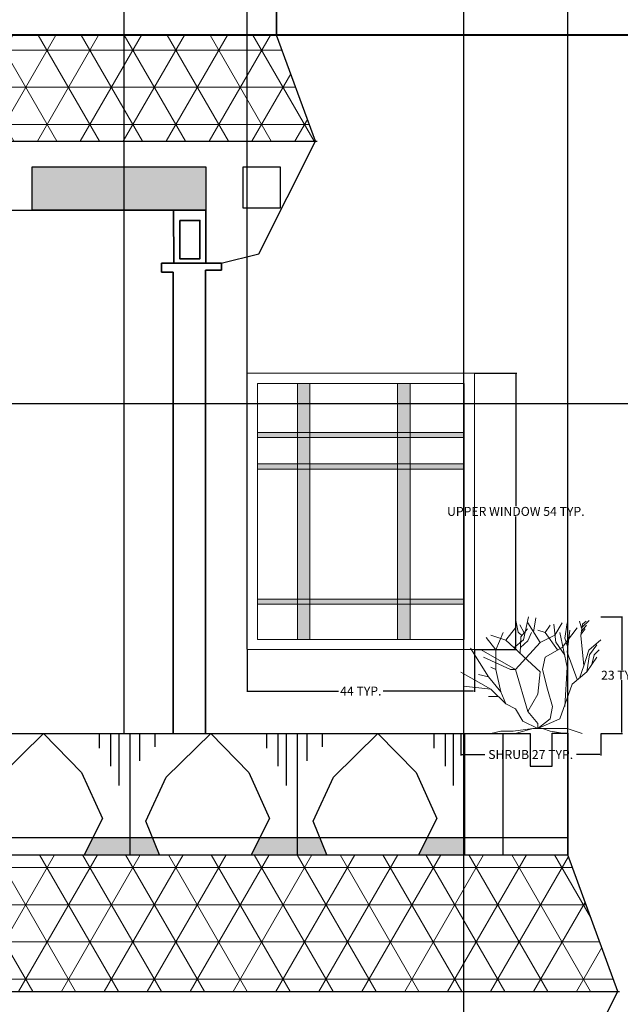
# Model space of a CAD drawing. Units: inches. Extents: x -17 to 741, y 7 to 490.
# Tile 5 of 8: x 371 to 489, y 191 to 383. Entities that reach past the tile are written whole.
import ezdxf

# ---------------------------------------------------------------- set-up
doc = ezdxf.new("R2010")
doc.units = ezdxf.units.IN
doc.header["$MEASUREMENT"] = 0
for name, color, linetype, lineweight in [('A-ANNO-DIMS', 2, 'Continuous', 18), ('A-COLS', 1, 'Continuous', 35), ('A-ELEV-PATT', 252, 'Continuous', 13), ('A-FLOR-RAIL', 7, 'Continuous', 25), ('A-GLAZ', 4, 'Continuous', 18), ('A-ROOF', 7, 'Continuous', 35), ('A-ROOF-CNPE', 7, 'Continuous', 25), ('A-ROOF-PATT', 8, 'Continuous', 13), ('A-WALL-TRIM', 7, 'Continuous', 25), ('L-PLNT', 3, 'Continuous', 18)]:
    doc.layers.add(name, color=color, linetype=linetype, lineweight=lineweight)
doc.styles.get("Standard").update_dxf_attribs({"font": 'arial.ttf'})
doc.dimstyles.get("Standard").update_dxf_attribs({"dimtxt": 1.75, "dimasz": 0.18, "dimexe": 0.18, "dimexo": 0.0625, "dimgap": 0.09, "dimtad": 0, "dimtih": 1, "dimtoh": 1, "dimdec": 4, "dimzin": 0, "dimdsep": 46, "dimlunit": 4, "dimtxsty": 'Standard', "dimcen": 0.09, "dimadec": 0, "dimazin": 0, "dimtfac": 1, "dimtdec": 4, "dimtofl": 0, "dimtmove": 0, "dimatfit": 3, "dimfxl": 1, "dimtolj": 1, "dimtzin": 0, "dimarcsym": 0})

# ---------------------------------------------------------------- blocks, each defined once
blk = doc.blocks.new('Shrub - elevation')
for p, q in [((-12.471, 19.775), (-12.898, 22.044)), ((-11.28, 19.619), (-12.104, 21.184)), ((-11.433, 18.289), (-10.457, 22.749)), ((-8.16, 17.76), (-10.56, 21.6)), ((-9.48, 19.775), (-8.992, 22.592)), ((-5.086, 17.741), (-5.513, 21.34)), ((-5.28, 19.2), (-3.84, 21.6)), ((-3.377, 18.602), (-2.888, 21.575)), ((-0.508, 21.888), (-0.081, 20.558)), ((-0.203, 19.149), (0.102, 21.34)), ((0.041, 20.714), (1.384, 22.044)), ((0.102, 21.34), (0.835, 21.888)), ((-16.8, 16.32), (-15.36, 19.68)), ((-14.88, 18.24), (-12.96, 20.64)), ((-11.677, 19.071), (-12.471, 19.775)), ((-11.921, 18.836), (-10.64, 20.401)), ((-10.579, 18.054), (-9.846, 19.697)), ((-7.2, 19.68), (-8.64, 20.16)), ((-7.2, 19.68), (-6.24, 21.12)), ((-4.8, 16.32), (-7.2, 19.68)), ((-2.88, 12.96), (-4.32, 19.68)), ((-3.84, 16.8), (-0.96, 20.64)), ((-2.88, 15.84), (-2.4, 20.16)), ((-0.142, 19.384), (0.59, 20.401)), ((-0.02, 20.01), (0.896, 21.105)), ((-16.8, 16.32), (-18.72, 18.72)), ((-14.88, 18.24), (-17.76, 19.2)), ((-8.16, 12), (-14.88, 18.24)), ((-13.325, 16.724), (-11.433, 18.289)), ((-12.96, 12.48), (-8.16, 17.76)), ((-12.043, 15.628), (-11.921, 18.836)), ((-11.982, 16.802), (-10.579, 18.054)), ((-8.16, 17.76), (-5.28, 19.2)), ((-3.377, 15.315), (-5.086, 17.819)), ((-2.766, 16.802), (-3.377, 18.602)), ((0.346, 13.203), (-0.203, 19.149)), ((1.323, 16.254), (3.642, 18.289)), ((-18.24, 11.04), (-21.755, 16.655)), ((-12.96, 12.48), (-19.68, 16.32)), ((-16.8, 12.48), (-16.8, 16.32)), ((-7.2, 14.88), (-3.84, 16.8)), ((-0.96, 10.56), (-2.88, 15.84)), ((0.346, 13.203), (1.323, 16.254)), ((1.44, 15.36), (2.88, 17.28)), ((2.4, 15.36), (3.36, 16.32)), ((-13.92, 12.48), (-19.2, 14.88)), ((-7.68, 12.48), (-7.2, 14.88)), ((0.96, 12), (1.44, 15.36)), ((0.96, 12), (2.88, 14.88)), ((1.92, 13.44), (2.4, 15.36)), ((-17.76, 8.64), (-23.663, 11.961)), ((-16.8, 12.48), (-17.76, 12.96)), ((-15.84, 8.16), (-16.8, 12.48)), ((-12.96, 12.48), (-13.92, 12.48)), ((-10.56, 4.32), (-12.96, 12.48)), ((-8.64, 7.68), (-8.16, 12)), ((-6.72, 8.64), (-7.68, 12.48)), ((-3.36, 5.28), (-2.88, 12.96)), ((-1.92, 9.6), (0.96, 12)), ((-0.48, 10.8), (0.346, 13.203)), ((-18.24, 11.04), (-20.16, 11.52)), ((-15.84, 8.16), (-18.24, 11.04)), ((-17.76, 8.64), (-23.128, 9.222)), ((-14.88, 5.76), (-17.76, 8.64)), ((-14.88, 5.76), (-15.84, 8.16)), ((-5.76, 5.28), (-6.72, 8.64)), ((-4.32, 2.88), (-1.92, 9.6)), ((-16.32, 7.2), (-18.24, 7.2)), ((-10.56, 4.32), (-8.64, 7.68)), ((-12.96, 4.8), (-14.88, 5.76)), ((-11.52, 2.4), (-12.96, 4.8)), ((-8.64, 1.92), (-10.56, 4.32)), ((-6.24, 2.88), (-5.76, 5.28)), ((-8.64, 0.96), (-11.52, 2.4)), ((-8.64, 0.96), (-4.32, 2.88)), ((-8.64, 0.96), (-6.24, 2.88)), ((-15.84, 0.48), (-17.76, 0)), ((-13.44, 0.48), (-15.84, 0.48)), ((-9.6, 0.96), (-13.44, 0.48)), ((-9.6, 0.96), (-12.96, 0)), ((-9.6, 0.96), (-7.68, 0.96)), ((-8.64, 0.96), (-8.64, 1.92)), ((-8.64, 0.96), (-2.88, 0.96)), ((-7.68, 0.96), (-6.24, 0.48)), ((-6.24, 0.48), (-3.36, 0)), ((-2.88, 0.96), (0, 0))]:
    blk.add_line(p, q)
blk = doc.blocks.new('BALCONY-POINTED-PANEL')
for p, q in [((0, 23.66), (33.75, 23.66)), ((1.12, 23.66), (1.12, 14.33)), ((2.97, 23.66), (2.97, 18.36)), ((6.01, 23.66), (6.01, 21.09)), ((27.76, 23.66), (27.76, 20.83)), ((29.99, 23.66), (29.99, 17.32)), ((31.57, 23.66), (31.57, 13.51)), ((33.75, 23.66), (33.75, 0))]:
    blk.add_line(p, q)
blk.add_lwpolyline([(6.92, 0), (4.23, 6.57), (8.17, 15.14), (16.88, 23.66), (24.3, 16.07), (28.38, 7.1), (24.8, 0)])
blk = doc.blocks.new('WIN-ELEV-DIVIDED')
for p, q in [((9.78, 51.92), (9.78, 2)), ((12.23, 51.92), (12.23, 2)), ((29.29, 51.92), (29.29, 2)), ((31.75, 51.92), (31.75, 2)), ((2, 42.35), (42.31, 42.35)), ((2, 41.35), (42.31, 41.35)), ((2, 36.22), (42.31, 36.22)), ((2, 35.22), (42.31, 35.22)), ((2, 9.85), (42.31, 9.85)), ((2, 8.85), (42.31, 8.85))]:
    blk.add_line(p, q)
for points in [[(0, 0), (44.31, 0), (44.31, 53.92), (0, 53.92)], [(2, 2), (42.31, 2), (42.31, 51.92), (2, 51.92)]]:
    blk.add_lwpolyline(points, close=True)
blk = doc.blocks.new('*D23')
at = {"layer": 'A-ANNO-DIMS', "color": 0, "lineweight": -2, "transparency": 16777216}
for p, q in [((460.15, 313.97), (468.35, 313.97)), ((468.17, 313.79), (468.17, 288)), ((468.17, 260.23), (468.17, 286.01)), ((460.15, 260.05), (468.35, 260.05))]:
    blk.add_line(p, q, dxfattribs=at)
at = {"layer": 'A-ANNO-DIMS', "color": 0, "transparency": 16777216}
for points in [[(468.14, 313.79), (468.2, 313.79), (468.17, 313.97)], [(468.14, 260.23), (468.2, 260.23), (468.17, 260.05)]]:
    blk.add_solid(points, dxfattribs=at)
at = {"layer": 'Defpoints', "color": 0, "transparency": 16777216}
for p in [(460.09, 313.97), (468.17, 313.97), (460.09, 260.05)]:
    blk.add_point(p, dxfattribs=at)
at = {"layer": 'A-ANNO-DIMS', "color": 0, "transparency": 16777216, "insert": (468.17, 287.01), "char_height": 1.75, "attachment_point": 5}
blk.add_mtext('\\A1;UPPER WINDOW 54 TYP.', dxfattribs=at)
blk = doc.blocks.new('*D24')
at = {"layer": 'A-ANNO-DIMS', "color": 0, "lineweight": -2, "transparency": 16777216}
for p, q in [((415.78, 259.99), (415.78, 251.78)), ((460.09, 259.99), (460.09, 251.78)), ((415.96, 251.96), (433.55, 251.96)), ((459.91, 251.96), (442.32, 251.96))]:
    blk.add_line(p, q, dxfattribs=at)
at = {"layer": 'A-ANNO-DIMS', "color": 0, "transparency": 16777216}
for points in [[(415.96, 251.99), (415.96, 251.93), (415.78, 251.96)], [(459.91, 251.99), (459.91, 251.93), (460.09, 251.96)]]:
    blk.add_solid(points, dxfattribs=at)
at = {"layer": 'Defpoints', "color": 0, "transparency": 16777216}
for p in [(415.78, 260.05), (460.09, 260.05), (460.09, 251.96)]:
    blk.add_point(p, dxfattribs=at)
at = {"layer": 'A-ANNO-DIMS', "color": 0, "transparency": 16777216, "insert": (437.93, 251.96), "char_height": 1.75, "attachment_point": 5}
blk.add_mtext('\\A1;44 TYP.', dxfattribs=at)
blk = doc.blocks.new('*D31')
at = {"layer": 'A-ANNO-DIMS', "color": 0, "lineweight": -2, "transparency": 16777216}
for p, q in [((457.41, 243.61), (457.41, 239.4)), ((484.72, 243.61), (484.72, 239.4)), ((457.59, 239.58), (462.1, 239.58)), ((484.54, 239.58), (480.03, 239.58))]:
    blk.add_line(p, q, dxfattribs=at)
at = {"layer": 'A-ANNO-DIMS', "color": 0, "transparency": 16777216}
for points in [[(457.59, 239.61), (457.59, 239.55), (457.41, 239.58)], [(484.54, 239.61), (484.54, 239.55), (484.72, 239.58)]]:
    blk.add_solid(points, dxfattribs=at)
at = {"layer": 'Defpoints', "color": 0, "transparency": 16777216}
for p in [(457.41, 243.68), (484.72, 243.68), (484.72, 239.58)]:
    blk.add_point(p, dxfattribs=at)
at = {"layer": 'A-ANNO-DIMS', "color": 0, "transparency": 16777216, "insert": (471.07, 239.58), "char_height": 1.75, "attachment_point": 5}
blk.add_mtext('\\A1;SHRUB 27 TYP.', dxfattribs=at)
blk = doc.blocks.new('*D32')
at = {"layer": 'A-ANNO-DIMS', "color": 0, "lineweight": -2, "transparency": 16777216}
for p, q in [((484.78, 266.43), (489, 266.43)), ((488.82, 266.25), (488.82, 256.04)), ((488.82, 243.86), (488.82, 254.07)), ((484.78, 243.68), (489, 243.68))]:
    blk.add_line(p, q, dxfattribs=at)
at = {"layer": 'A-ANNO-DIMS', "color": 0, "transparency": 16777216}
for points in [[(488.79, 266.25), (488.85, 266.25), (488.82, 266.43)], [(488.79, 243.86), (488.85, 243.86), (488.82, 243.68)]]:
    blk.add_solid(points, dxfattribs=at)
at = {"layer": 'Defpoints', "color": 0, "transparency": 16777216}
for p in [(484.72, 266.43), (488.82, 266.43), (484.72, 243.68)]:
    blk.add_point(p, dxfattribs=at)
at = {"layer": 'A-ANNO-DIMS', "color": 0, "transparency": 16777216, "insert": (488.82, 255.05), "char_height": 1.75, "attachment_point": 5}
blk.add_mtext('\\A1;23 TYP.', dxfattribs=at)
blk = doc.blocks.new('*D37')
at = {"layer": 'A-ANNO-DIMS', "color": 0, "lineweight": -2, "transparency": 16777216}
for p, q in [((20.52, 396.95), (20.52, 14.58)), ((553.43, 51.95), (553.43, 14.58)), ((20.7, 14.76), (283.93, 14.76)), ((553.25, 14.76), (290.02, 14.76))]:
    blk.add_line(p, q, dxfattribs=at)
at = {"layer": 'A-ANNO-DIMS', "color": 0, "transparency": 16777216}
for points in [[(20.7, 14.79), (20.7, 14.73), (20.52, 14.76)], [(553.25, 14.79), (553.25, 14.73), (553.43, 14.76)]]:
    blk.add_solid(points, dxfattribs=at)
at = {"layer": 'Defpoints', "color": 0, "transparency": 16777216}
for p in [(20.52, 397.01), (553.43, 52.01), (553.43, 14.76)]:
    blk.add_point(p, dxfattribs=at)
at = {"layer": 'A-ANNO-DIMS', "color": 0, "transparency": 16777216, "insert": (286.97, 14.76), "char_height": 1.75, "attachment_point": 5}
blk.add_mtext('\\A1;532.9', dxfattribs=at)
blk = doc.blocks.new('*D38')
at = {"layer": 'A-ANNO-DIMS', "color": 0, "lineweight": -2, "transparency": 16777216}
for p, q in [((341.83, 454.57), (723.06, 454.57)), ((722.88, 454.39), (722.88, 254.27)), ((722.88, 52.19), (722.88, 252.31)), ((553.49, 52.01), (723.06, 52.01))]:
    blk.add_line(p, q, dxfattribs=at)
at = {"layer": 'A-ANNO-DIMS', "color": 0, "transparency": 16777216}
for points in [[(722.85, 454.39), (722.91, 454.39), (722.88, 454.57)], [(722.85, 52.19), (722.91, 52.19), (722.88, 52.01)]]:
    blk.add_solid(points, dxfattribs=at)
at = {"layer": 'Defpoints', "color": 0, "transparency": 16777216}
for p in [(341.77, 454.57), (722.88, 454.57), (553.43, 52.01)]:
    blk.add_point(p, dxfattribs=at)
at = {"layer": 'A-ANNO-DIMS', "color": 0, "transparency": 16777216, "insert": (722.88, 253.29), "char_height": 1.75, "attachment_point": 5}
blk.add_mtext('\\A1;402.6', dxfattribs=at)
blk = doc.blocks.new('*D47')
at = {"layer": 'A-ANNO-DIMS', "color": 0, "lineweight": -2, "transparency": 16777216}
for p, q in [((493.03, 379.95), (-13.46, 379.95)), ((-13.28, 379.77), (-13.28, 344.94)), ((-13.28, 308.15), (-13.28, 342.97)), ((553.37, 307.97), (-13.46, 307.97))]:
    blk.add_line(p, q, dxfattribs=at)
at = {"layer": 'A-ANNO-DIMS', "color": 0, "transparency": 16777216}
for points in [[(-13.31, 379.77), (-13.25, 379.77), (-13.28, 379.95)], [(-13.31, 308.15), (-13.25, 308.15), (-13.28, 307.97)]]:
    blk.add_solid(points, dxfattribs=at)
at = {"layer": 'Defpoints', "color": 0, "transparency": 16777216}
for p in [(493.1, 379.95), (-13.28, 307.97), (553.43, 307.97)]:
    blk.add_point(p, dxfattribs=at)
at = {"layer": 'A-ANNO-DIMS', "color": 0, "transparency": 16777216, "insert": (-13.28, 343.96), "char_height": 1.75, "attachment_point": 5}
blk.add_mtext('\\A1;71.98', dxfattribs=at)
blk = doc.blocks.new('*D53')
at = {"layer": 'A-ANNO-DIMS', "color": 0, "lineweight": -2, "transparency": 16777216}
for p, q in [((271.44, 167.89), (271.44, 488.55)), ((271.62, 488.37), (361.78, 488.37)), ((457.87, 488.37), (367.7, 488.37)), ((458.05, 167.89), (458.05, 488.55))]:
    blk.add_line(p, q, dxfattribs=at)
at = {"layer": 'A-ANNO-DIMS', "color": 0, "transparency": 16777216}
for points in [[(271.62, 488.4), (271.62, 488.34), (271.44, 488.37)], [(457.87, 488.4), (457.87, 488.34), (458.05, 488.37)]]:
    blk.add_solid(points, dxfattribs=at)
at = {"layer": 'Defpoints', "color": 0, "transparency": 16777216}
for p in [(458.05, 488.37), (271.44, 167.83), (458.05, 167.83)]:
    blk.add_point(p, dxfattribs=at)
at = {"layer": 'A-ANNO-DIMS', "color": 0, "transparency": 16777216, "insert": (364.74, 488.37), "char_height": 1.75, "attachment_point": 5}
blk.add_mtext('\\A1;186.6', dxfattribs=at)
blk = doc.blocks.new('*D54')
at = {"layer": 'A-ANNO-DIMS', "color": 0, "lineweight": -2, "transparency": 16777216}
for p, q in [((458.05, 167.89), (458.05, 488.55)), ((458.23, 488.37), (502.69, 488.37)), ((553.25, 488.37), (508.78, 488.37)), ((553.43, 52.07), (553.43, 488.55))]:
    blk.add_line(p, q, dxfattribs=at)
at = {"layer": 'A-ANNO-DIMS', "color": 0, "transparency": 16777216}
for points in [[(458.23, 488.4), (458.23, 488.34), (458.05, 488.37)], [(553.25, 488.4), (553.25, 488.34), (553.43, 488.37)]]:
    blk.add_solid(points, dxfattribs=at)
at = {"layer": 'Defpoints', "color": 0, "transparency": 16777216}
for p in [(553.43, 488.37), (458.05, 167.83), (553.43, 52.01)]:
    blk.add_point(p, dxfattribs=at)
at = {"layer": 'A-ANNO-DIMS', "color": 0, "transparency": 16777216, "insert": (505.74, 488.37), "char_height": 1.75, "attachment_point": 5}
blk.add_mtext('\\A1;95.38', dxfattribs=at)
blk = doc.blocks.new('*D57')
at = {"layer": 'A-ANNO-DIMS', "color": 0, "lineweight": -2, "transparency": 16777216}
for p, q in [((325.44, 243.73), (325.44, 488.55)), ((325.62, 488.37), (367.57, 488.37)), ((415.6, 488.37), (373.65, 488.37)), ((415.78, 260.11), (415.78, 488.55))]:
    blk.add_line(p, q, dxfattribs=at)
at = {"layer": 'A-ANNO-DIMS', "color": 0, "transparency": 16777216}
for points in [[(325.62, 488.4), (325.62, 488.34), (325.44, 488.37)], [(415.6, 488.4), (415.6, 488.34), (415.78, 488.37)]]:
    blk.add_solid(points, dxfattribs=at)
at = {"layer": 'Defpoints', "color": 0, "transparency": 16777216}
for p in [(415.78, 488.37), (415.78, 260.05), (325.44, 243.67)]:
    blk.add_point(p, dxfattribs=at)
at = {"layer": 'A-ANNO-DIMS', "color": 0, "transparency": 16777216, "insert": (370.61, 488.37), "char_height": 1.75, "attachment_point": 5}
blk.add_mtext('\\A1;90.34', dxfattribs=at)
blk = doc.blocks.new('*D65')
at = {"layer": 'A-ANNO-DIMS', "color": 0, "lineweight": -2, "transparency": 16777216}
for p, q in [((478.32, 220.07), (478.32, 488.55)), ((478.5, 488.37), (513.01, 488.37)), ((553.25, 488.37), (518.74, 488.37)), ((553.43, 308.03), (553.43, 488.55))]:
    blk.add_line(p, q, dxfattribs=at)
at = {"layer": 'A-ANNO-DIMS', "color": 0, "transparency": 16777216}
for points in [[(478.5, 488.4), (478.5, 488.34), (478.32, 488.37)], [(553.25, 488.4), (553.25, 488.34), (553.43, 488.37)]]:
    blk.add_solid(points, dxfattribs=at)
at = {"layer": 'Defpoints', "color": 0, "transparency": 16777216}
for p in [(553.43, 488.37), (553.43, 307.97), (478.32, 220.01)]:
    blk.add_point(p, dxfattribs=at)
at = {"layer": 'A-ANNO-DIMS', "color": 0, "transparency": 16777216, "insert": (515.87, 488.37), "char_height": 1.75, "attachment_point": 5}
blk.add_mtext('\\A1;75.11', dxfattribs=at)
blk = doc.blocks.new('*D67')
at = {"layer": 'A-ANNO-DIMS', "color": 0, "lineweight": -2, "transparency": 16777216}
for p, q in [((359.14, 243.73), (359.14, 488.55)), ((359.32, 488.37), (372.41, 488.37)), ((391.59, 488.37), (378.49, 488.37)), ((391.77, 243.73), (391.77, 488.55))]:
    blk.add_line(p, q, dxfattribs=at)
at = {"layer": 'A-ANNO-DIMS', "color": 0, "transparency": 16777216}
for points in [[(359.32, 488.4), (359.32, 488.34), (359.14, 488.37)], [(391.59, 488.4), (391.59, 488.34), (391.77, 488.37)]]:
    blk.add_solid(points, dxfattribs=at)
at = {"layer": 'Defpoints', "color": 0, "transparency": 16777216}
for p in [(391.77, 488.37), (359.14, 243.67), (391.77, 243.67)]:
    blk.add_point(p, dxfattribs=at)
at = {"layer": 'A-ANNO-DIMS', "color": 0, "transparency": 16777216, "insert": (375.45, 488.37), "char_height": 1.75, "attachment_point": 5}
blk.add_mtext('\\A1;32.63', dxfattribs=at)

msp = doc.modelspace()

# ---------------------------------------------------------------- hatches: boundary and pattern name
at = {"layer": 'A-ELEV-PATT'}
h = msp.add_hatch(dxfattribs=at)
h.set_pattern_fill('STARS', color=256, scale=19)
h.paths.add_polyline_path([(204.6793, 330.2905), (174.1219, 330.2905), (174.1219, 324.7204), (204.6793, 324.7204)])
h.paths.add_polyline_path([(238.7618, 330.6251), (208.2044, 330.6251), (208.2044, 325.055), (238.7618, 325.055)])
h.paths.add_polyline_path([(316.4391, 354.2167), (282.5434, 354.2167), (282.5434, 345.7496), (316.4391, 345.7496)])
h.paths.add_polyline_path([(360.3395, 354.2167), (326.4438, 354.2167), (326.4438, 345.7496), (360.3395, 345.7496)])
h.paths.add_polyline_path([(407.6938, 354.2167), (373.7981, 354.2167), (373.7981, 345.7496), (407.6938, 345.7496)])
h.paths.add_polyline_path([(290.7055, 188.3373), (256.8098, 188.3373), (256.8098, 179.8702), (290.7055, 179.8702)])
h.paths.add_polyline_path([(332.372, 188.3373), (298.4763, 188.3373), (298.4763, 179.8702), (332.372, 179.8702)])
h.paths.add_polyline_path([(375.4339, 188.3373), (341.5382, 188.3373), (341.5382, 179.8702), (375.4339, 179.8702)])
h.paths.add_polyline_path([(419.3343, 188.3373), (385.4386, 188.3373), (385.4386, 179.8702), (419.3343, 179.8702)])
h.paths.add_polyline_path([(466.6886, 188.3373), (432.7929, 188.3373), (432.7929, 179.8702), (466.6886, 179.8702)])
h = msp.add_hatch(color=256, dxfattribs=at)
h.dxf.hatch_style = 1
h.paths.add_polyline_path([(323.0665, 158.6389), (301.7867, 158.6389), (301.7867, 78.0082), (323.0665, 78.0082)])
h.paths.add_polyline_path([(318.3825, 145.2592), (318.3825, 85.0354), (307.7462, 85.0354), (307.7462, 145.2592)], flags=16)
h.paths.add_polyline_path([(344.3462, 158.6389), (323.0665, 158.6389), (323.0665, 78.0082), (344.3462, 78.0082)])
h.paths.add_polyline_path([(339.3004, 145.2592), (339.3004, 85.0354), (328.6642, 85.0354), (328.6642, 145.2592)], flags=16)
h.paths.add_polyline_path([(192.7233, 151.6028), (190.2672, 151.6028), (190.2672, 142.0361), (192.7233, 142.0361)])
h.paths.add_polyline_path([(192.7233, 141.0361), (190.2672, 141.0361), (190.2672, 135.6738), (192.7233, 135.6738)])
h.paths.add_polyline_path([(192.7233, 142.0361), (190.2672, 142.0361), (190.2672, 141.0361), (192.7233, 141.0361)])
h.paths.add_polyline_path([(209.3698, 142.0361), (192.7233, 142.0361), (192.7233, 141.0361), (209.3698, 141.0361)])
h.paths.add_polyline_path([(190.2672, 142.0361), (183.5379, 142.0361), (183.5379, 141.0361), (190.2672, 141.0361)])
h.paths.add_polyline_path([(190.2672, 135.6738), (183.5379, 135.6738), (183.5379, 134.6738), (190.2672, 134.6738)])
h.paths.add_polyline_path([(192.7233, 135.6738), (190.2672, 135.6738), (190.2672, 134.6738), (192.7233, 134.6738)])
h.paths.add_polyline_path([(192.7233, 134.6738), (190.2672, 134.6738), (190.2672, 101.6848), (192.7233, 101.6848)])
h.paths.add_polyline_path([(209.3698, 135.6738), (192.7233, 135.6738), (192.7233, 134.6738), (209.3698, 134.6738)])
h.paths.add_polyline_path([(211.8259, 135.6738), (209.3698, 135.6738), (209.3698, 134.6738), (211.8259, 134.6738)])
h.paths.add_polyline_path([(211.8259, 141.0361), (209.3698, 141.0361), (209.3698, 135.6738), (211.8259, 135.6738)])
h.paths.add_polyline_path([(211.8259, 142.0361), (209.3698, 142.0361), (209.3698, 141.0361), (211.8259, 141.0361)])
h.paths.add_polyline_path([(211.8259, 151.6028), (209.3698, 151.6028), (209.3698, 142.0361), (211.8259, 142.0361)])
h.paths.add_polyline_path([(223.8474, 142.0361), (211.8259, 142.0361), (211.8259, 141.0361), (223.8474, 141.0361)])
h.paths.add_polyline_path([(223.8474, 135.6738), (211.8259, 135.6738), (211.8259, 134.6738), (223.8474, 134.6738)])
h.paths.add_polyline_path([(211.8259, 134.6738), (209.3698, 134.6738), (209.3698, 108.8153), (211.8259, 108.8153)])
h.paths.add_polyline_path([(211.8259, 108.8153), (209.3698, 108.8153), (209.3698, 107.8153), (211.8259, 107.8153)])
h.paths.add_polyline_path([(211.8259, 107.8153), (209.3698, 107.8153), (209.3698, 101.6848), (211.8259, 101.6848)])
h.paths.add_polyline_path([(223.8474, 108.8153), (211.8259, 108.8153), (211.8259, 107.8153), (223.8474, 107.8153)])
h.paths.add_polyline_path([(209.3698, 108.8153), (192.7233, 108.8153), (192.7233, 107.8153), (209.3698, 107.8153)])
h.paths.add_polyline_path([(190.2672, 108.8153), (183.5379, 108.8153), (183.5379, 107.8153), (190.2672, 107.8153)])
h.paths.add_polyline_path([(147.2864, 151.6028), (144.8304, 151.6028), (144.8304, 109.315), (147.2864, 109.315)])
h.paths.add_polyline_path([(147.2864, 109.315), (144.8304, 109.315), (144.8304, 108.315), (147.2864, 108.315)])
h.paths.add_polyline_path([(147.2864, 108.315), (144.8304, 108.315), (144.8304, 101.6848), (147.2864, 101.6848)])
h.paths.add_polyline_path([(157.8499, 109.315), (147.2864, 109.315), (147.2864, 108.315), (157.8499, 108.315)])
h.paths.add_polyline_path([(144.8304, 109.315), (127.7745, 109.315), (127.7745, 108.315), (144.8304, 108.315)])
h.paths.add_polyline_path([(127.7745, 109.315), (125.3184, 109.315), (125.3184, 108.315), (127.7745, 108.315)])
h.paths.add_polyline_path([(127.7745, 151.6028), (125.3184, 151.6028), (125.3184, 109.315), (127.7745, 109.315)])
h.paths.add_polyline_path([(125.3184, 109.315), (117.5405, 109.315), (117.5405, 108.315), (125.3184, 108.315)])
h.paths.add_polyline_path([(127.7745, 108.315), (125.3184, 108.315), (125.3184, 101.6848), (127.7745, 101.6848)])
h.paths.add_polyline_path([(125.3184, 135.9009), (117.5405, 135.9009), (117.5405, 134.9009), (125.3184, 134.9009)])
h.paths.add_polyline_path([(144.8304, 135.9009), (127.7745, 135.9009), (127.7745, 134.9009), (144.8304, 134.9009)])
h.paths.add_polyline_path([(157.8499, 135.9009), (147.2864, 135.9009), (147.2864, 134.9009), (157.8499, 134.9009)])
h.paths.add_polyline_path([(144.8304, 142.0361), (127.7745, 142.0361), (127.7745, 141.0361), (144.8304, 141.0361)])
h.paths.add_polyline_path([(157.8499, 142.0361), (147.2864, 142.0361), (147.2864, 141.0361), (157.8499, 141.0361)])
h.paths.add_polyline_path([(125.3184, 142.0361), (117.5405, 142.0361), (117.5405, 141.0361), (125.3184, 141.0361)])
h.paths.add_polyline_path([(447.5234, 311.9659), (445.0673, 311.9659), (445.0673, 302.3991), (447.5234, 302.3991)])
h.paths.add_polyline_path([(447.5234, 302.3991), (445.0673, 302.3991), (445.0673, 301.3991), (447.5234, 301.3991)])
h.paths.add_polyline_path([(458.0869, 302.3991), (447.5234, 302.3991), (447.5234, 301.3991), (458.0869, 301.3991)])
h.paths.add_polyline_path([(447.5234, 301.3991), (445.0673, 301.3991), (445.0673, 296.2639), (447.5234, 296.2639)])
h.paths.add_polyline_path([(447.5234, 296.2639), (445.0673, 296.2639), (445.0673, 295.2639), (447.5234, 295.2639)])
h.paths.add_polyline_path([(458.0869, 296.2639), (447.5234, 296.2639), (447.5234, 295.2639), (458.0869, 295.2639)])
h.paths.add_polyline_path([(445.0673, 296.2639), (428.0115, 296.2639), (428.0115, 295.2639), (445.0673, 295.2639)])
h.paths.add_polyline_path([(447.5234, 295.2639), (445.0673, 295.2639), (445.0673, 262.0479), (447.5234, 262.0479)])
h.paths.add_polyline_path([(445.0673, 302.3991), (428.0115, 302.3991), (428.0115, 301.3991), (445.0673, 301.3991)])
h.paths.add_polyline_path([(428.0115, 302.3991), (425.5554, 302.3991), (425.5554, 301.3991), (428.0115, 301.3991)])
h.paths.add_polyline_path([(428.0115, 311.9659), (425.5554, 311.9659), (425.5554, 302.3991), (428.0115, 302.3991)])
h.paths.add_polyline_path([(425.5554, 302.3991), (417.7774, 302.3991), (417.7774, 301.3991), (425.5554, 301.3991)])
h.paths.add_polyline_path([(428.0115, 301.3991), (425.5554, 301.3991), (425.5554, 296.2639), (428.0115, 296.2639)])
h.paths.add_polyline_path([(425.5554, 296.2639), (417.7774, 296.2639), (417.7774, 295.2639), (425.5554, 295.2639)])
h.paths.add_polyline_path([(428.0115, 296.2639), (425.5554, 296.2639), (425.5554, 295.2639), (428.0115, 295.2639)])
h.paths.add_polyline_path([(428.0115, 295.2639), (425.5554, 295.2639), (425.5554, 262.0479), (428.0115, 262.0479)])
h.paths.add_polyline_path([(425.5554, 269.8939), (417.7774, 269.8939), (417.7774, 268.8939), (425.5554, 268.8939)])
h.paths.add_polyline_path([(445.0673, 269.8939), (428.0115, 269.8939), (428.0115, 268.8939), (445.0673, 268.8939)])
h.paths.add_polyline_path([(458.0869, 269.8939), (447.5234, 269.8939), (447.5234, 268.8939), (458.0869, 268.8939)])
h = msp.add_hatch(color=256, dxfattribs=at)
h.dxf.hatch_style = 1
h.paths.add_polyline_path([(103.6141, 223.3801), (98.075, 223.3801), (98.075, 220.0082), (104.992, 220.0082)])
h.paths.add_polyline_path([(131.8275, 223.3801), (124.5765, 223.3801), (122.878, 220.0082), (131.8275, 220.0082)])
h.paths.add_polyline_path([(136.2468, 223.3801), (131.8275, 223.3801), (131.8275, 220.0082), (137.6247, 220.0082)])
h.paths.add_polyline_path([(164.4602, 223.3801), (157.2092, 223.3801), (155.5107, 220.0082), (164.4602, 220.0082)])
h.paths.add_polyline_path([(168.8795, 223.3801), (164.4602, 223.3801), (164.4602, 220.0082), (170.2574, 220.0082)])
h.paths.add_polyline_path([(197.0929, 223.3801), (189.8419, 223.3801), (188.1434, 220.0082), (197.0929, 220.0082)])
h.paths.add_polyline_path([(201.5121, 223.3801), (197.0929, 223.3801), (197.0929, 220.0082), (202.8901, 220.0082)])
h.paths.add_polyline_path([(229.7256, 223.3801), (222.4746, 223.3801), (220.776, 220.0082), (229.7256, 220.0082)])
h.paths.add_polyline_path([(234.1448, 223.3801), (229.7256, 223.3801), (229.7256, 220.0082), (235.5227, 220.0082)])
h.paths.add_polyline_path([(262.3583, 223.3801), (255.1072, 223.3801), (253.4087, 220.0082), (262.3583, 220.0082)])
h.paths.add_polyline_path([(266.7775, 223.3801), (262.3583, 223.3801), (262.3583, 220.0082), (268.1554, 220.0082)])
h.paths.add_polyline_path([(294.9909, 223.3801), (287.7399, 223.3801), (286.0414, 220.0082), (294.9909, 220.0082)])
h.paths.add_polyline_path([(299.4102, 223.3801), (294.9909, 223.3801), (294.9909, 220.0082), (300.7881, 220.0082)])
h.paths.add_polyline_path([(327.6236, 223.3801), (320.3726, 223.3801), (318.6741, 220.0082), (327.6236, 220.0082)])
h.paths.add_polyline_path([(332.0429, 223.3801), (327.6236, 223.3801), (327.6236, 220.0082), (333.4208, 220.0082)])
h.paths.add_polyline_path([(360.2563, 223.3801), (353.0053, 223.3801), (351.3068, 220.0082), (360.2563, 220.0082)])
h.paths.add_polyline_path([(364.6755, 223.3801), (360.2563, 223.3801), (360.2563, 220.0082), (361.2234, 220.0082), (366.0535, 220.0082)])
h.paths.add_polyline_path([(392.889, 223.3801), (385.638, 223.3801), (383.9394, 220.0082), (392.889, 220.0082)])
h.paths.add_polyline_path([(397.3082, 223.3801), (392.889, 223.3801), (392.889, 220.0082), (398.6861, 220.0082)])
h.paths.add_polyline_path([(425.5216, 223.3801), (418.2706, 223.3801), (416.5721, 220.0082), (425.5216, 220.0082)])
h.paths.add_polyline_path([(429.9409, 223.3801), (425.5216, 223.3801), (425.5216, 220.0082), (431.3188, 220.0082)])
h.paths.add_polyline_path([(458.1543, 223.3801), (450.9033, 223.3801), (449.2048, 220.0082), (458.1543, 220.0082)])
at = {"layer": 'A-ROOF-PATT'}
h = msp.add_hatch(dxfattribs=at)
h.set_pattern_fill('NET3', color=256, scale=58)
h.paths.add_polyline_path([(478.3168, 220.0082), (470.3932, 220.0082), (361.2234, 220.0082), (239.9367, 220.0082), (229.7523, 193.3539), (470.754, 193.3539), (488.0578, 193.3539)])
h.paths.add_polyline_path([(421.4932, 379.9466), (278.7803, 379.9466), (278.7803, 359.2334), (411.7592, 359.2334), (429.063, 359.2334)])

# ---------------------------------------------------------------- linework, layer by layer
at = {"layer": 'A-COLS'}
for p, q in [((401.428, 335.4124), (401.3756, 345.7496)), ((401.428, 335.4124), (401.3756, 345.7496)), ((407.6938, 335.4124), (407.6938, 345.7496)), ((407.6938, 335.4124), (407.6938, 345.7496)), ((399.0546, 333.7049), (399.0546, 335.4124)), ((399.0546, 335.4124), (410.7317, 335.4124)), ((399.0546, 333.7049), (399.0546, 335.4124)), ((399.0546, 335.4124), (410.7317, 335.4124)), ((410.7317, 335.4124), (410.7317, 334.0843)), ((410.7317, 335.4124), (410.7317, 334.0843)), ((401.3072, 333.7049), (399.0546, 333.7049)), ((401.3072, 333.7049), (399.0546, 333.7049)), ((401.3072, 327.0147), (401.3072, 333.7049)), ((401.3072, 327.0147), (401.3072, 333.7049)), ((410.7317, 334.0843), (407.666, 334.0843)), ((407.666, 334.0843), (407.666, 329.7221)), ((410.7317, 334.0843), (407.666, 334.0843)), ((407.666, 334.0843), (407.666, 329.7221)), ((407.666, 243.669), (407.666, 329.7221)), ((407.666, 243.669), (407.666, 329.7221)), ((401.3072, 279.0657), (401.3072, 327.0147)), ((401.3072, 279.0657), (401.3072, 327.0147)), ((401.3072, 279.0657), (401.3072, 243.669))]:
    msp.add_line(p, q, dxfattribs=at)
msp.add_lwpolyline([(402.6265, 343.7805), (406.5568, 343.7805), (406.5568, 336.3002), (402.6265, 336.3002)], close=True, dxfattribs=at)
msp.add_lwpolyline([(402.6265, 343.7805), (406.5568, 343.7805), (406.5568, 336.3002), (402.6265, 336.3002)], close=True, dxfattribs=at)
at = {"layer": 'A-FLOR-RAIL'}
for p, q in [((458.1543, 243.669), (465.6209, 243.669)), ((465.6209, 243.669), (465.6209, 220.0082)), ((465.6209, 243.669), (470.983, 243.669)), ((470.983, 243.669), (470.983, 237.3273)), ((475.2726, 237.3273), (475.2726, 243.7567)), ((475.2726, 243.7567), (478.3168, 243.7567)), ((478.3168, 243.7567), (478.3168, 220.0082)), ((470.983, 237.3273), (475.2726, 237.3273)), ((98.075, 223.3801), (478.3168, 223.3801))]:
    msp.add_line(p, q, dxfattribs=at)
at = {"layer": 'A-ROOF'}
msp.add_line((421.4932, 379.9466), (421.4932, 387.669), dxfattribs=at)
at = {"layer": 'A-ROOF-CNPE'}
for p, q in [((411.3984, 359.2334), (429.4238, 359.2334)), ((411.3984, 359.2334), (429.4238, 359.2334)), ((278.7803, 345.7496), (407.6938, 345.7496)), ((278.7803, 345.7496), (407.6938, 345.7496)), ((470.3932, 220.0082), (478.3168, 220.0082)), ((470.3932, 193.3539), (488.4186, 193.3539))]:
    msp.add_line(p, q, dxfattribs=at)
for points in [[(429.063, 359.2334), (421.4932, 379.9466)], [(429.063, 359.2334), (421.4932, 379.9466)], [(278.7803, 359.2334), (411.7592, 359.2334)], [(278.7803, 359.2334), (411.7592, 359.2334)], [(410.7038, 335.4124), (418.0483, 337.2783), (429.063, 359.2334)], [(410.7038, 335.4124), (418.0483, 337.2783), (429.063, 359.2334)], [(239.9367, 220.0082), (229.7523, 193.3539), (470.754, 193.3539)], [(361.2234, 220.0082), (470.3932, 220.0082)], [(488.0578, 193.3539), (478.3168, 220.0082)], [(469.6986, 169.533), (477.0431, 171.3989), (488.0578, 193.3539)]]:
    msp.add_lwpolyline(points, dxfattribs=at)
for points in [[(373.7981, 354.2167), (407.6938, 354.2167), (407.6938, 345.7496), (373.7981, 345.7496)], [(373.7981, 354.2167), (407.6938, 354.2167), (407.6938, 345.7496), (373.7981, 345.7496)], [(414.9873, 354.2167), (422.1817, 354.2167), (422.1817, 346.1773), (414.9873, 346.1773)], [(414.9873, 354.2167), (422.1817, 354.2167), (422.1817, 346.1773), (414.9873, 346.1773)]]:
    msp.add_lwpolyline(points, close=True, dxfattribs=at)
at = {"layer": 'A-WALL-TRIM'}
msp.add_lwpolyline([(53.4591, 295.9), (53.4591, 295.9), (72.6093, 295.9), (97.1425, 365.3552), (97.1425, 379.9466), (515.96, 379.9466)], dxfattribs=at)

# ---------------------------------------------------------------- block references
at = {"layer": 'A-FLOR-RAIL'}
for p in [(359.1364, 220.008), (391.7691, 220.008), (424.4018, 220.008)]:
    msp.add_blockref('BALCONY-POINTED-PANEL', p, dxfattribs=at)
at = {"layer": 'A-GLAZ'}
msp.add_blockref('WIN-ELEV-DIVIDED', (415.7774, 260.048), dxfattribs=at)
at = {"layer": 'L-PLNT'}
msp.add_blockref('Shrub - elevation', (481.0777, 243.6767), dxfattribs=at)

# ---------------------------------------------------------------- dimensions: what is measured, and where the dimension line sits
at = {"layer": 'A-ANNO-DIMS'}
for base, p1, p2, override, picture, middle in [((458.0494, 488.3717), (271.4367, 167.8255), (458.0494, 167.8255), {"dimdec": 1, "dimlfac": 1, "dimrnd": 0, "dimzin": 0, "dimdsep": 46, "dimlunit": 2}, '*D53', (364.743, 488.3717)), ((415.7774, 488.3717), (325.441, 243.669), (415.7774, 260.0479), {"dimdec": 2, "dimlfac": 1, "dimrnd": 0, "dimzin": 0, "dimdsep": 46, "dimlunit": 2}, '*D57', (370.6092, 488.3717)), ((391.7691, 488.3717), (359.1364, 243.669), (391.7691, 243.669), {"dimdec": 2, "dimlfac": 1, "dimrnd": 0, "dimzin": 0, "dimdsep": 46, "dimlunit": 2}, '*D67', (375.4527, 488.3717)), ((553.4286, 488.3717), (458.0494, 167.8255), (553.4286, 52.0082), {"dimdec": 2, "dimlfac": 1, "dimrnd": 0, "dimzin": 0, "dimdsep": 46, "dimlunit": 2}, '*D54', (505.739, 488.3717)), ((553.4286, 488.3717), (478.3168, 220.0082), (553.4286, 307.9703), {"dimdec": 2, "dimlfac": 1, "dimrnd": 0, "dimzin": 0, "dimdsep": 46, "dimlunit": 2}, '*D65', (515.8727, 488.3717)), ((553.4286, 14.7597), (20.5169, 397.0087), (553.4286, 52.0082), {"dimdec": 1, "dimlfac": 1, "dimrnd": 0, "dimzin": 0, "dimdsep": 46, "dimlunit": 2}, '*D37', (286.9727, 14.7597))]:
    dim = msp.add_linear_dim(base=base, p1=p1, p2=p2, dimstyle='Standard', override=override, dxfattribs=at)
    dim.commit()
    dim.dimension.update_dxf_attribs({"geometry": picture, "text_midpoint": middle})
for base, p1, p2, override, picture, middle in [((722.8826, 454.5717), (553.4286, 52.0082), (341.7687, 454.5717), {"dimdec": 1, "dimlfac": 1, "dimrnd": 0, "dimzin": 0, "dimdsep": 46, "dimlunit": 2}, '*D38', (722.8826, 253.2899)), ((-13.2831, 307.9703), (493.0961, 379.9466), (553.4286, 307.9703), {"dimdec": 2, "dimlfac": 1, "dimrnd": 0, "dimzin": 0, "dimdsep": 46, "dimlunit": 2}, '*D47', (-13.2831, 343.9584))]:
    dim = msp.add_linear_dim(base=base, p1=p1, p2=p2, angle=90, dimstyle='Standard', override=override, dxfattribs=at)
    dim.commit()
    dim.dimension.update_dxf_attribs({"geometry": picture, "text_midpoint": middle})
for base, p1, p2, text, picture, middle in [((468.1746, 313.9659), (460.0869, 260.0479), (460.0869, 313.9659), 'UPPER WINDOW <> TYP.', '*D23', (468.1746, 287.0069)), ((488.8154, 266.4257), (484.7197, 243.6767), (484.7197, 266.4257), '<> TYP.', '*D32', (488.8154, 255.0512))]:
    dim = msp.add_linear_dim(base=base, p1=p1, p2=p2, angle=90, text=text, dimstyle='Standard', override={"dimdec": 0, "dimlfac": 1, "dimrnd": 0, "dimzin": 0, "dimdsep": 46, "dimlunit": 2}, dxfattribs=at)
    dim.commit()
    dim.dimension.update_dxf_attribs({"geometry": picture, "text_midpoint": middle})
for base, p1, p2, text, picture, middle in [((460.0869, 251.9602), (415.7774, 260.0479), (460.0869, 260.0479), '<> TYP.', '*D24', (437.9322, 251.9602)), ((484.7197, 239.581), (457.4147, 243.6767), (484.7197, 243.6767), 'SHRUB <> TYP.', '*D31', (471.0672, 239.581))]:
    dim = msp.add_linear_dim(base=base, p1=p1, p2=p2, text=text, dimstyle='Standard', override={"dimdec": 0, "dimlfac": 1, "dimrnd": 0, "dimzin": 0, "dimdsep": 46, "dimlunit": 2}, dxfattribs=at)
    dim.commit()
    dim.dimension.update_dxf_attribs({"geometry": picture, "text_midpoint": middle})

doc.saveas('drawing.dxf')
